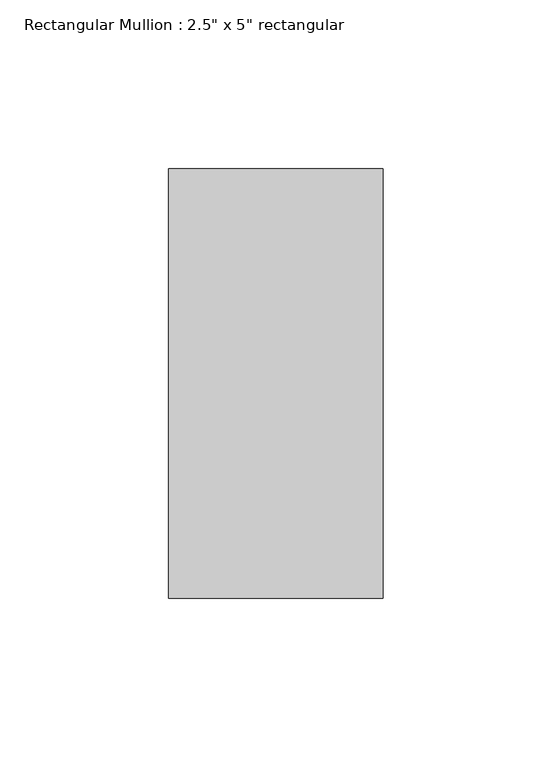
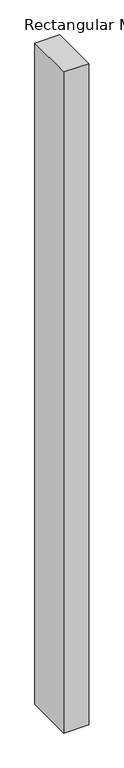
"""IFC4 building model written with IfcOpenShell, lengths in millimetres: member geometry."""

from ifc_helpers import new_model, si_unit, frame, origin, place, context, project, spatial, polyline, outline, extrude, source, transform, mapped, element, save


def member_6a3d3fef(model_context):
    return source(origin(), model_context, "Body", "SweptSolid", [
        extrude(outline(polyline([(0.0, 63.5), (0.0, -63.5), (-63.5, -63.5), (-63.5, 63.5), (0.0, 63.5)])), frame((0.0, 0.0, -1777.3307027), z_axis=(0.0, 0.0, 1.0), x_axis=(1.0, 0.0, 0.0)), (0.0, 0.0, 1.0), 1777.3307027),
    ])


if __name__ == "__main__":
    model = new_model("IFC4")
    model_context = context("Model", 3, world=origin())
    ifc_project = project(units=[si_unit("LENGTHUNIT", "METRE", prefix="MILLI")], contexts=[model_context])
    site = spatial("IfcSite", under=ifc_project)
    building = spatial("IfcBuilding", under=site)
    placement = place(None, origin())
    member_shape = member_6a3d3fef(model_context)
    element("IfcMember", 1, ObjectType="Rectangular Mullion : 2.5\" x 5\" rectangular", at=placement, inside=building, context=model_context, shape_type="MappedRepresentation", body=[
        mapped(member_shape, transform((0.0, 0.0, 0.0), x_axis=(1.0, 0.0, 0.0), y_axis=(0.0, 1.0, 0.0), z_axis=(0.0, 0.0, 1.0))),
    ])
    save(model, "model.ifc")

# Revit data of these elements
# Type "Rectangular Mullion : 2.5\" x 5\" rectangular"
#   built-in parameter 1007304 = 0.416667 (stored number, unit not read)
#   built-in parameter 1007301 = 0.104167 (stored number, unit not read)
#   built-in parameter 1007300 = 0.104167 (stored number, unit not read)
# Element 1 (IfcMember, "Rectangular Mullion : 2.5\" x 5\" rectangular")
#   Materials on its faces: "Aluminum"
# Materials
#   "Aluminum": class "Metal", colour RGB 247 247 247, transparency 0, Description = "Aluminum 6061", Cost = 0
